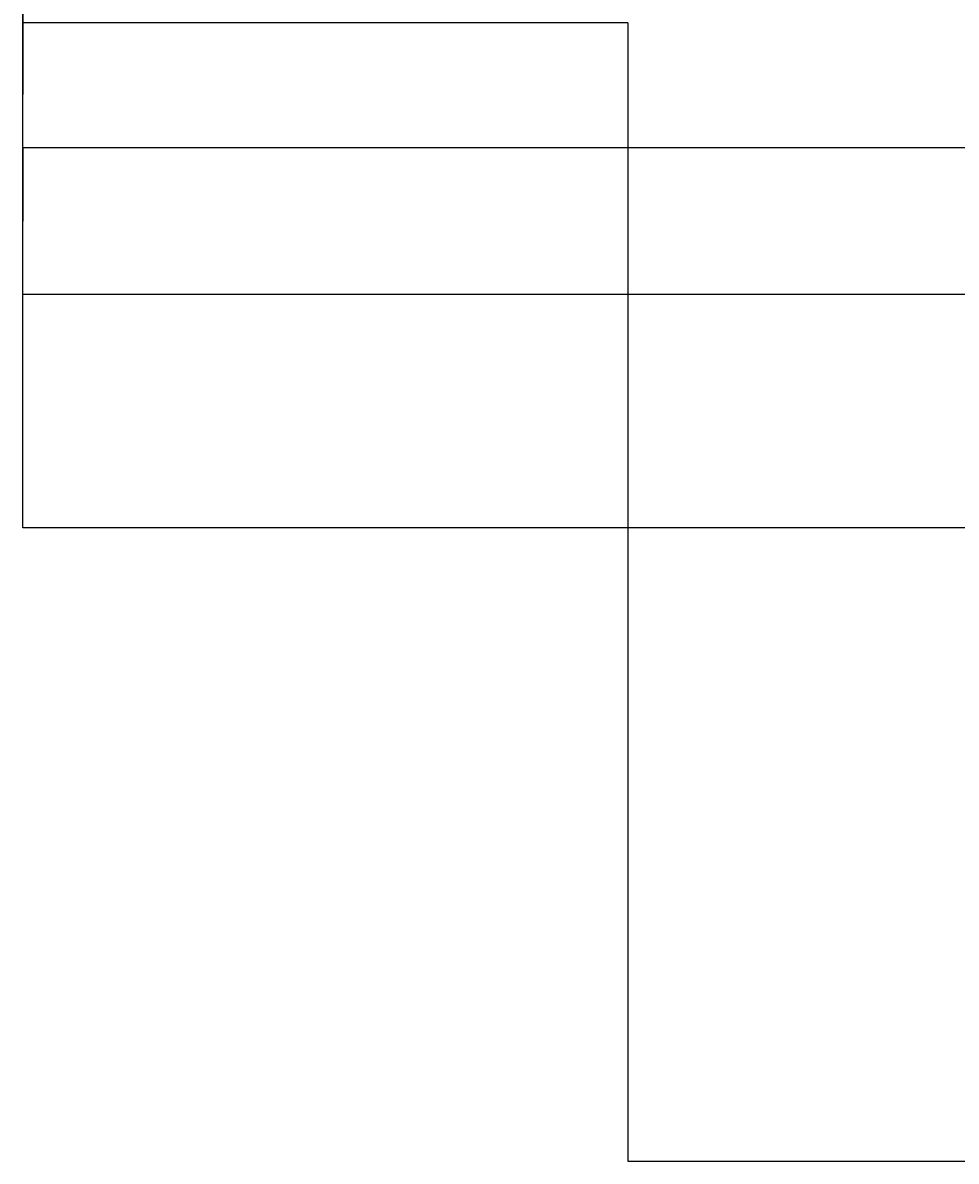
# Model space of a CAD drawing. Units: inches. Extents: x 35362 to 73946, y 43607 to 67532.
# Tile 1 of 134: x 35362 to 38077, y 43607 to 46919. Entities that reach past the tile are written whole.
import ezdxf

# ---------------------------------------------------------------- set-up
doc = ezdxf.new("R2010")
doc.units = ezdxf.units.IN
doc.header["$MEASUREMENT"] = 0
doc.layers.add('A-ANNO-DIMS', color=2, linetype='Continuous', lineweight=18)
doc.styles.get("Standard").update_dxf_attribs({"font": 'arial.ttf'})
doc.dimstyles.get("Standard").update_dxf_attribs({"dimtxt": 0.18, "dimasz": 0.18, "dimexe": 0.18, "dimexo": 0.0625, "dimgap": 0.09, "dimtad": 0, "dimtih": 1, "dimtoh": 1, "dimdec": 4, "dimzin": 0, "dimdsep": 46, "dimtxsty": 'Standard', "dimcen": 0.09, "dimadec": 0, "dimazin": 0, "dimtfac": 1, "dimtdec": 4, "dimtofl": 0, "dimtmove": 0, "dimatfit": 3, "dimfxl": 1, "dimtolj": 1, "dimtzin": 0, "dimarcsym": 0})

# ---------------------------------------------------------------- blocks, each defined once
blk = doc.blocks.new('*D5')
at = {"layer": 'A-ANNO-DIMS', "color": 0, "lineweight": -2, "transparency": 16777216}
for p, q in [((37121.9, 46919.3), (37121.9, 43606.7)), ((69871.5, 45449.8), (69871.5, 43606.7)), ((37122.1, 43606.9), (53496.3, 43606.9)), ((69871.3, 43606.9), (53497.2, 43606.9))]:
    blk.add_line(p, q, dxfattribs=at)
at = {"layer": 'A-ANNO-DIMS', "color": 0, "transparency": 16777216}
for points in [[(37122.1, 43606.9), (37122.1, 43606.8), (37121.9, 43606.9)], [(69871.3, 43606.9), (69871.3, 43606.8), (69871.5, 43606.9)]]:
    blk.add_solid(points, dxfattribs=at)
at = {"layer": 'Defpoints', "color": 0, "transparency": 16777216}
for p in [(37121.9, 46919.4), (69871.5, 45449.9), (69871.5, 43606.9)]:
    blk.add_point(p, dxfattribs=at)
at = {"layer": 'A-ANNO-DIMS', "color": 0, "transparency": 16777216, "insert": (53496.7, 43606.9), "char_height": 0.18, "attachment_point": 5}
blk.add_mtext('\\A1;32750', dxfattribs=at)
blk = doc.blocks.new('*D15')
at = {"layer": 'A-ANNO-DIMS', "color": 0, "lineweight": -2, "transparency": 16777216}
for p, q in [((37121.9, 46919.3), (37121.9, 43606.7)), ((39894.8, 46919.3), (39894.8, 43606.7)), ((37122.1, 43606.9), (38508, 43606.9)), ((39894.7, 43606.9), (38508.8, 43606.9))]:
    blk.add_line(p, q, dxfattribs=at)
at = {"layer": 'A-ANNO-DIMS', "color": 0, "transparency": 16777216}
for points in [[(37122.1, 43606.9), (37122.1, 43606.8), (37121.9, 43606.9)], [(39894.7, 43606.9), (39894.7, 43606.8), (39894.8, 43606.9)]]:
    blk.add_solid(points, dxfattribs=at)
at = {"layer": 'Defpoints', "color": 0, "transparency": 16777216}
for p in [(37121.9, 46919.4), (39894.8, 46919.4), (39894.8, 43606.9)]:
    blk.add_point(p, dxfattribs=at)
at = {"layer": 'A-ANNO-DIMS', "color": 0, "transparency": 16777216, "insert": (38508.4, 43606.9), "char_height": 0.18, "attachment_point": 5}
blk.add_mtext('\\A1;2773', dxfattribs=at)
blk = doc.blocks.new('*D16')
at = {"layer": 'A-ANNO-DIMS', "color": 0, "lineweight": -2, "transparency": 16777216}
for p, q in [((37121.9, 49689.8), (35361.8, 49689.8)), ((35361.9, 49689.7), (35361.9, 48304.8)), ((35361.9, 46919.6), (35361.9, 48304.4)), ((37121.9, 46919.4), (35361.8, 46919.4))]:
    blk.add_line(p, q, dxfattribs=at)
at = {"layer": 'A-ANNO-DIMS', "color": 0, "transparency": 16777216}
for points in [[(35361.9, 49689.7), (35362, 49689.7), (35361.9, 49689.8)], [(35361.9, 46919.6), (35362, 46919.6), (35361.9, 46919.4)]]:
    blk.add_solid(points, dxfattribs=at)
at = {"layer": 'Defpoints', "color": 0, "transparency": 16777216}
for p in [(37121.9, 49689.8), (35361.9, 46919.4), (37121.9, 46919.4)]:
    blk.add_point(p, dxfattribs=at)
at = {"layer": 'A-ANNO-DIMS', "color": 0, "transparency": 16777216, "insert": (35361.9, 48304.6), "char_height": 0.18, "attachment_point": 5}
blk.add_mtext('\\A1;2770.5', dxfattribs=at)
blk = doc.blocks.new('*D67')
at = {"layer": 'A-ANNO-DIMS', "color": 0, "lineweight": -2, "transparency": 16777216}
for p, q in [((56873.5, 53351.5), (35361.8, 53351.5)), ((35361.9, 53351.3), (35361.9, 49400.9)), ((35361.9, 45450.1), (35361.9, 49400.5)), ((53793.6, 45449.9), (35361.8, 45449.9))]:
    blk.add_line(p, q, dxfattribs=at)
at = {"layer": 'A-ANNO-DIMS', "color": 0, "transparency": 16777216}
for points in [[(35361.9, 53351.3), (35362, 53351.3), (35361.9, 53351.5)], [(35361.9, 45450.1), (35362, 45450.1), (35361.9, 45449.9)]]:
    blk.add_solid(points, dxfattribs=at)
at = {"layer": 'Defpoints', "color": 0, "transparency": 16777216}
for p in [(35361.9, 53351.5), (56873.6, 53351.5), (53793.6, 45449.9)]:
    blk.add_point(p, dxfattribs=at)
at = {"layer": 'A-ANNO-DIMS', "color": 0, "transparency": 16777216, "insert": (35361.9, 49400.7), "char_height": 0.18, "attachment_point": 5}
blk.add_mtext('\\A1;7901.6', dxfattribs=at)
blk = doc.blocks.new('*D76')
at = {"layer": 'A-ANNO-DIMS', "color": 0, "lineweight": -2, "transparency": 16777216}
for p, q in [((54052.8, 46555.3), (35361.8, 46555.3)), ((35361.9, 46555.1), (35361.9, 46342.3)), ((35361.9, 46129.1), (35361.9, 46341.9)), ((53793.6, 46128.9), (35361.8, 46128.9))]:
    blk.add_line(p, q, dxfattribs=at)
at = {"layer": 'A-ANNO-DIMS', "color": 0, "transparency": 16777216}
for points in [[(35361.9, 46555.1), (35362, 46555.1), (35361.9, 46555.3)], [(35361.9, 46129.1), (35362, 46129.1), (35361.9, 46128.9)]]:
    blk.add_solid(points, dxfattribs=at)
at = {"layer": 'Defpoints', "color": 0, "transparency": 16777216}
for p in [(35361.9, 46555.3), (54052.9, 46555.3), (53793.6, 46128.9)]:
    blk.add_point(p, dxfattribs=at)
at = {"layer": 'A-ANNO-DIMS', "color": 0, "transparency": 16777216, "insert": (35361.9, 46342.1), "char_height": 0.18, "attachment_point": 5}
blk.add_mtext('\\A1;426.4', dxfattribs=at)
blk = doc.blocks.new('*D90')
at = {"layer": 'A-ANNO-DIMS', "color": 0, "lineweight": -2, "transparency": 16777216}
for p, q in [((53707.7, 47291.3), (35361.8, 47291.3)), ((35361.9, 47291.1), (35361.9, 46710.3)), ((35361.9, 46129.1), (35361.9, 46709.9)), ((53793.6, 46128.9), (35361.8, 46128.9))]:
    blk.add_line(p, q, dxfattribs=at)
at = {"layer": 'A-ANNO-DIMS', "color": 0, "transparency": 16777216}
for points in [[(35361.9, 47291.1), (35362, 47291.1), (35361.9, 47291.3)], [(35361.9, 46129.1), (35362, 46129.1), (35361.9, 46128.9)]]:
    blk.add_solid(points, dxfattribs=at)
at = {"layer": 'Defpoints', "color": 0, "transparency": 16777216}
for p in [(53707.8, 47291.3), (35361.9, 46128.9), (53793.6, 46128.9)]:
    blk.add_point(p, dxfattribs=at)
at = {"layer": 'A-ANNO-DIMS', "color": 0, "transparency": 16777216, "insert": (35361.9, 46710.1), "char_height": 0.18, "attachment_point": 5}
blk.add_mtext('\\A1;1162.4', dxfattribs=at)

msp = doc.modelspace()

# ---------------------------------------------------------------- dimensions: what is measured, and where the dimension line sits
at = {"layer": 'A-ANNO-DIMS'}
for base, p1, p2, picture, middle in [((35361.949, 53351.529), (53793.638, 45449.894), (56873.602, 53351.529), '*D67', (35361.949, 49400.712)), ((35361.949, 46919.381), (37121.949, 49689.843), (37121.949, 46919.381), '*D16', (35361.949, 48304.612)), ((35361.949, 46128.878), (53707.781, 47291.285), (53793.638, 46128.878), '*D90', (35361.949, 46710.081)), ((35361.949, 46555.293), (53793.638, 46128.878), (54052.899, 46555.293), '*D76', (35361.949, 46342.086))]:
    dim = msp.add_linear_dim(base=base, p1=p1, p2=p2, angle=90, dimstyle='Standard', override={"dimdec": 1, "dimlfac": 1, "dimrnd": 0, "dimzin": 0, "dimdsep": 46, "dimlunit": 2}, dxfattribs=at)
    dim.commit()
    dim.dimension.update_dxf_attribs({"geometry": picture, "text_midpoint": middle})
for base, p2, picture, middle in [((69871.496, 43606.859), (69871.496, 45449.894), '*D5', (53496.723, 43606.859)), ((39894.84, 43606.859), (39894.84, 46919.381), '*D15', (38508.395, 43606.859))]:
    dim = msp.add_linear_dim(base=base, p1=(37121.949, 46919.381), p2=p2, dimstyle='Standard', override={"dimdec": 0, "dimlfac": 1, "dimrnd": 0, "dimzin": 0, "dimdsep": 46, "dimlunit": 2}, dxfattribs=at)
    dim.commit()
    dim.dimension.update_dxf_attribs({"geometry": picture, "text_midpoint": middle})

doc.saveas('drawing.dxf')
